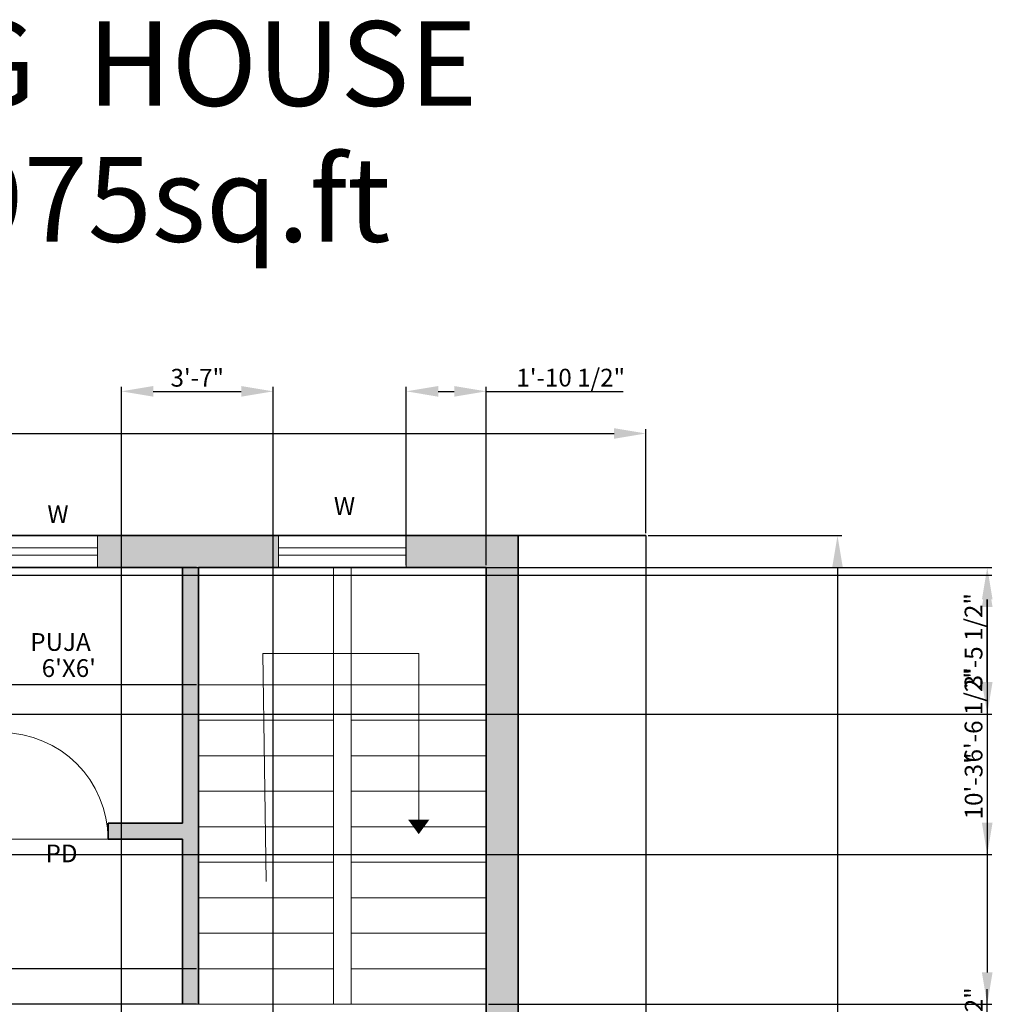
# Model space of a CAD drawing. Units: inches. Extents: x 2265 to 2807, y 1544 to 2401.
# Tile 9 of 9: x 2531 to 2807, y 2124 to 2401. Entities that reach past the tile are written whole.
import ezdxf

# ---------------------------------------------------------------- set-up
doc = ezdxf.new("R2010")
doc.units = ezdxf.units.IN
for name, color, linetype, lineweight in [('A-ANNO-DIMS', 2, 'Continuous', 18), ('A-ANNO-TEXT', 7, 'Continuous', 18), ('A-ANNO-TITL', 7, 'Continuous', 35), ('A-AREA-IDEN', 7, 'Continuous', 18), ('A-DOOR', 3, 'Continuous', 18), ('A-FLOR-STRS', 7, 'Continuous', 18), ('A-GLAZ', 4, 'Continuous', 18), ('A-WALL', 7, 'Continuous', 35), ('A-WALL-PATT', 18, 'Continuous', 13), ('C-PROP', 7, 'Continuous', 25)]:
    doc.layers.add(name, color=color, linetype=linetype, lineweight=lineweight)
doc.styles.add('ARIAL', font='times.ttf', dxfattribs={"height": 5})
doc.styles.get("Standard").update_dxf_attribs({"font": 'arial.ttf', "height": 5})
doc.dimstyles.new('ISO-25', dxfattribs={"dimtxt": 5, "dimasz": 9, "dimexe": 1.25, "dimexo": 0.625, "dimtad": 1, "dimlunit": 3, "dimtxsty": 'Standard', "dimcen": 2.5, "dimadec": 0, "dimazin": 0, "dimtfac": 1, "dimtmove": 0, "dimatfit": 3, "dimfxl": 1, "dimarcsym": 0})

# ---------------------------------------------------------------- blocks, each defined once
blk = doc.blocks.new('*D5')
at = {"layer": 'A-ANNO-DIMS', "color": 0, "lineweight": -2, "transparency": 16777216}
for p, q in [((2323.1, 2256.36), (2323.1, 2285.73)), ((2707.1, 2256.36), (2707.1, 2285.73)), ((2332.1, 2284.48), (2698.1, 2284.48))]:
    blk.add_line(p, q, dxfattribs=at)
at = {"layer": 'A-ANNO-DIMS', "color": 0, "lineweight": 100, "transparency": 16777216}
for points in [[(2332.1, 2285.98), (2332.1, 2282.98), (2323.1, 2284.48)], [(2698.1, 2285.98), (2698.1, 2282.98), (2707.1, 2284.48)]]:
    blk.add_solid(points, dxfattribs=at)
at = {"layer": 'Defpoints', "color": 0, "lineweight": 100, "transparency": 16777216}
for p in [(2707.1, 2284.48), (2323.1, 2255.73), (2707.1, 2255.73)]:
    blk.add_point(p, dxfattribs=at)
at = {"layer": 'A-ANNO-DIMS', "color": 0, "transparency": 16777216, "insert": (2515.1, 2287.66), "char_height": 5, "attachment_point": 5}
blk.add_mtext("32'", dxfattribs=at)
blk = doc.blocks.new('*D6')
at = {"layer": 'A-ANNO-DIMS', "color": 0, "lineweight": -2, "transparency": 16777216}
for p, q in [((2707.73, 2255.73), (2762.29, 2255.73)), ((2761.04, 2246.73), (2761.04, 1814.73)), ((2707.73, 1805.73), (2762.29, 1805.73))]:
    blk.add_line(p, q, dxfattribs=at)
at = {"layer": 'A-ANNO-DIMS', "color": 0, "lineweight": 100, "transparency": 16777216}
for points in [[(2759.54, 2246.73), (2762.54, 2246.73), (2761.04, 2255.73)], [(2759.54, 1814.73), (2762.54, 1814.73), (2761.04, 1805.73)]]:
    blk.add_solid(points, dxfattribs=at)
at = {"layer": 'Defpoints', "color": 0, "lineweight": 100, "transparency": 16777216}
for p in [(2707.1, 2255.73), (2707.1, 1805.73), (2761.04, 1805.73)]:
    blk.add_point(p, dxfattribs=at)
at = {"layer": 'A-ANNO-DIMS', "color": 0, "transparency": 16777216, "insert": (2757.86, 2030.73), "char_height": 5, "attachment_point": 5, "rotation": 90}
blk.add_mtext('37\'-6"', dxfattribs=at)
blk = doc.blocks.new('GLAZING-36IN')
for p, q in [((0, 36), (0, 0)), ((3.5, 36), (3.5, 0)), ((5.5, 36), (5.5, 0)), ((5.5, 36), (5.5, 0)), ((9, 0), (9, 36))]:
    blk.add_line(p, q)
blk = doc.blocks.new('GLAZING-24IN')
for p, q in [((0, 24), (0, 0)), ((3.5, 24), (3.5, 0)), ((5.5, 24), (5.5, 0)), ((5.5, 24), (5.5, 0)), ((9, 0), (9, 24))]:
    blk.add_line(p, q)
blk = doc.blocks.new('DOOR-SWING-30IN')
for p, q in [((2, 29.93), (2, 0)), ((0, 0), (30, 0))]:
    blk.add_line(p, q)
blk.add_arc((0, 0), 30, 0, 90)
blk = doc.blocks.new('*D36')
at = {"layer": 'A-ANNO-DIMS', "color": 0, "lineweight": -2, "transparency": 16777216}
for p, q in [((2662.73, 2246.73), (2804.46, 2246.73)), ((2803.21, 2237.73), (2803.21, 2132.73)), ((2662.73, 2123.73), (2804.46, 2123.73))]:
    blk.add_line(p, q, dxfattribs=at)
at = {"layer": 'A-ANNO-DIMS', "color": 0, "lineweight": 100, "transparency": 16777216}
for points in [[(2801.71, 2237.73), (2804.71, 2237.73), (2803.21, 2246.73)], [(2801.71, 2132.73), (2804.71, 2132.73), (2803.21, 2123.73)]]:
    blk.add_solid(points, dxfattribs=at)
at = {"layer": 'Defpoints', "color": 0, "lineweight": 100, "transparency": 16777216}
for p in [(2662.1, 2246.73), (2662.1, 2123.73), (2803.21, 2123.73)]:
    blk.add_point(p, dxfattribs=at)
at = {"layer": 'A-ANNO-DIMS', "color": 0, "transparency": 16777216, "insert": (2800.03, 2185.23), "char_height": 5, "attachment_point": 5, "rotation": 90}
blk.add_mtext('10\'-3"', dxfattribs=at)
blk = doc.blocks.new('*D46')
at = {"layer": 'A-ANNO-DIMS', "color": 0, "lineweight": -2, "transparency": 16777216}
for p, q in [((2803.21, 2104.95), (2803.21, 2128.02)), ((2381.23, 2095.95), (2804.46, 2095.95)), ((2803.21, 2082.06), (2803.21, 2095.95)), ((2381.23, 2082.06), (2804.46, 2082.06)), ((2803.21, 2073.06), (2803.21, 2064.06))]:
    blk.add_line(p, q, dxfattribs=at)
at = {"layer": 'A-ANNO-DIMS', "color": 0, "lineweight": 100, "transparency": 16777216}
for points in [[(2801.71, 2104.95), (2804.71, 2104.95), (2803.21, 2095.95)], [(2801.71, 2073.06), (2804.71, 2073.06), (2803.21, 2082.06)]]:
    blk.add_solid(points, dxfattribs=at)
at = {"layer": 'Defpoints', "color": 0, "lineweight": 100, "transparency": 16777216}
for p in [(2380.61, 2095.95), (2803.21, 2095.95), (2380.61, 2082.06)]:
    blk.add_point(p, dxfattribs=at)
at = {"layer": 'A-ANNO-DIMS', "color": 0, "transparency": 16777216, "insert": (2800.07, 2120.99), "char_height": 5, "attachment_point": 5, "rotation": 90}
blk.add_mtext('1\'-2"', dxfattribs=at)
blk = doc.blocks.new('*D51')
at = {"layer": 'A-ANNO-DIMS', "color": 0, "lineweight": -2, "transparency": 16777216}
for p, q in [((2470.16, 2244.62), (2804.46, 2244.62)), ((2803.21, 2235.62), (2803.21, 2174.88)), ((2466.22, 2165.88), (2804.46, 2165.88))]:
    blk.add_line(p, q, dxfattribs=at)
at = {"layer": 'A-ANNO-DIMS', "color": 0, "lineweight": 100, "transparency": 16777216}
for points in [[(2801.71, 2235.62), (2804.71, 2235.62), (2803.21, 2244.62)], [(2801.71, 2174.88), (2804.71, 2174.88), (2803.21, 2165.88)]]:
    blk.add_solid(points, dxfattribs=at)
at = {"layer": 'Defpoints', "color": 0, "lineweight": 100, "transparency": 16777216}
for p in [(2469.53, 2244.62), (2465.6, 2165.88), (2803.21, 2165.88)]:
    blk.add_point(p, dxfattribs=at)
at = {"layer": 'A-ANNO-DIMS', "color": 0, "transparency": 16777216, "insert": (2800, 2205.25), "char_height": 5, "attachment_point": 5, "rotation": 90}
blk.add_mtext('6\'-6 1/2"', dxfattribs=at)
blk = doc.blocks.new('*D52')
at = {"layer": 'A-ANNO-DIMS', "color": 0, "lineweight": -2, "transparency": 16777216}
for p, q in [((2559.35, 1939.86), (2559.35, 2297.59)), ((2568.35, 2296.34), (2593.1, 2296.34)), ((2602.1, 1939.86), (2602.1, 2297.59))]:
    blk.add_line(p, q, dxfattribs=at)
at = {"layer": 'A-ANNO-DIMS', "color": 0, "lineweight": 100, "transparency": 16777216}
for points in [[(2568.35, 2297.84), (2568.35, 2294.84), (2559.35, 2296.34)], [(2593.1, 2297.84), (2593.1, 2294.84), (2602.1, 2296.34)]]:
    blk.add_solid(points, dxfattribs=at)
at = {"layer": 'Defpoints', "color": 0, "lineweight": 100, "transparency": 16777216}
for p in [(2602.1, 2296.34), (2559.35, 1939.23), (2602.1, 1939.23)]:
    blk.add_point(p, dxfattribs=at)
at = {"layer": 'A-ANNO-DIMS', "color": 0, "transparency": 16777216, "insert": (2580.73, 2299.52), "char_height": 5, "attachment_point": 5}
blk.add_mtext('3\'-7"', dxfattribs=at)
blk = doc.blocks.new('*D56')
at = {"layer": 'A-ANNO-DIMS', "color": 0, "lineweight": -2, "transparency": 16777216}
for p, q in [((2639.6, 2247.36), (2639.6, 2297.59)), ((2648.6, 2296.34), (2653.1, 2296.34)), ((2662.1, 2247.36), (2662.1, 2297.59)), ((2662.1, 2296.34), (2700.71, 2296.34))]:
    blk.add_line(p, q, dxfattribs=at)
at = {"layer": 'A-ANNO-DIMS', "color": 0, "lineweight": 100, "transparency": 16777216}
for points in [[(2648.6, 2297.84), (2648.6, 2294.84), (2639.6, 2296.34)], [(2653.1, 2297.84), (2653.1, 2294.84), (2662.1, 2296.34)]]:
    blk.add_solid(points, dxfattribs=at)
at = {"layer": 'Defpoints', "color": 0, "lineweight": 100, "transparency": 16777216}
for p in [(2662.1, 2296.34), (2639.6, 2246.73), (2662.1, 2246.73)]:
    blk.add_point(p, dxfattribs=at)
at = {"layer": 'A-ANNO-DIMS', "color": 0, "transparency": 16777216, "insert": (2685.9, 2299.55), "char_height": 5, "attachment_point": 5}
blk.add_mtext('1\'-10 1/2"', dxfattribs=at)
blk = doc.blocks.new('*D57')
at = {"layer": 'A-ANNO-DIMS', "color": 0, "lineweight": -2, "transparency": 16777216}
for p, q in [((2368.73, 2246.73), (2804.46, 2246.73)), ((2803.21, 2214.48), (2803.21, 2237.73)), ((2368.73, 2205.48), (2804.46, 2205.48))]:
    blk.add_line(p, q, dxfattribs=at)
at = {"layer": 'A-ANNO-DIMS', "color": 0, "lineweight": 100, "transparency": 16777216}
for points in [[(2801.71, 2237.73), (2804.71, 2237.73), (2803.21, 2246.73)], [(2801.71, 2214.48), (2804.71, 2214.48), (2803.21, 2205.48)]]:
    blk.add_solid(points, dxfattribs=at)
at = {"layer": 'Defpoints', "color": 0, "lineweight": 100, "transparency": 16777216}
for p in [(2368.1, 2246.73), (2803.21, 2246.73), (2368.1, 2205.48)]:
    blk.add_point(p, dxfattribs=at)
at = {"layer": 'A-ANNO-DIMS', "color": 0, "transparency": 16777216, "insert": (2800, 2226.11), "char_height": 5, "attachment_point": 5, "rotation": 90}
blk.add_mtext('3\'-5 1/2"', dxfattribs=at)
blk = doc.blocks.new('*D59')
at = {"layer": 'A-ANNO-DIMS', "color": 0, "lineweight": -2, "transparency": 16777216}
for p, q in [((2580.48, 2246.73), (2274.04, 2246.73)), ((2275.29, 2237.73), (2275.29, 2222.73)), ((2580.48, 2213.73), (2274.04, 2213.73))]:
    blk.add_line(p, q, dxfattribs=at)
at = {"layer": 'A-ANNO-DIMS', "color": 0, "lineweight": 100, "transparency": 16777216}
for points in [[(2273.79, 2237.73), (2276.79, 2237.73), (2275.29, 2246.73)], [(2273.79, 2222.73), (2276.79, 2222.73), (2275.29, 2213.73)]]:
    blk.add_solid(points, dxfattribs=at)
at = {"layer": 'Defpoints', "color": 0, "lineweight": 100, "transparency": 16777216}
for p in [(2581.1, 2246.73), (2275.29, 2213.73), (2581.1, 2213.73)]:
    blk.add_point(p, dxfattribs=at)
at = {"layer": 'A-ANNO-DIMS', "color": 0, "transparency": 16777216, "insert": (2272.11, 2230.23), "char_height": 5, "attachment_point": 5, "rotation": 90}
blk.add_mtext('2\'-9"', dxfattribs=at)
blk = doc.blocks.new('*D60')
at = {"layer": 'A-ANNO-DIMS', "color": 0, "lineweight": -2, "transparency": 16777216}
for p, q in [((2275.29, 2142.73), (2275.29, 2151.73)), ((2580.48, 2133.73), (2274.04, 2133.73)), ((2275.29, 2133.73), (2275.29, 2123.73)), ((2580.48, 2123.73), (2274.04, 2123.73)), ((2275.29, 2114.73), (2275.29, 2087.31))]:
    blk.add_line(p, q, dxfattribs=at)
at = {"layer": 'A-ANNO-DIMS', "color": 0, "lineweight": 100, "transparency": 16777216}
for points in [[(2273.79, 2142.73), (2276.79, 2142.73), (2275.29, 2133.73)], [(2273.79, 2114.73), (2276.79, 2114.73), (2275.29, 2123.73)]]:
    blk.add_solid(points, dxfattribs=at)
at = {"layer": 'Defpoints', "color": 0, "lineweight": 100, "transparency": 16777216}
for p in [(2581.1, 2133.73), (2275.29, 2123.73), (2581.1, 2123.73)]:
    blk.add_point(p, dxfattribs=at)
at = {"layer": 'A-ANNO-DIMS', "color": 0, "transparency": 16777216, "insert": (2272.11, 2096.52), "char_height": 5, "attachment_point": 5, "rotation": 90}
blk.add_mtext('0\'-10"', dxfattribs=at)

msp = doc.modelspace()

# ---------------------------------------------------------------- hatches: boundary and pattern name
at = {"layer": 'A-WALL-PATT'}
h = msp.add_hatch(color=256, dxfattribs=at)
h.dxf.hatch_style = 1
h.paths.add_polyline_path([(2416.101, 2255.733), (2359.101, 2255.733), (2359.101, 2205.483), (2368.101, 2205.483), (2368.101, 2246.733), (2416.101, 2246.733)])
h.paths.add_polyline_path([(2528.601, 2255.733), (2452.101, 2255.733), (2452.101, 2246.733), (2487.251, 2246.733), (2500.101, 2246.733), (2500.101, 2168.733), (2504.601, 2168.733), (2504.601, 2170.233), (2525.601, 2170.233), (2525.601, 2174.733), (2504.601, 2174.733), (2504.601, 2246.733), (2528.601, 2246.733)])
h.paths.add_polyline_path([(2603.601, 2255.733), (2552.601, 2255.733), (2552.601, 2246.733), (2576.601, 2246.733), (2576.601, 2174.733), (2555.601, 2174.733), (2555.601, 2170.233), (2576.601, 2170.233), (2576.601, 2123.733), (2581.101, 2123.733), (2581.101, 2246.733), (2603.601, 2246.733)])
h.paths.add_polyline_path([(2671.101, 2255.733), (2639.601, 2255.733), (2639.601, 2246.733), (2662.101, 2246.733), (2662.101, 2083.435), (2671.101, 2083.435)])
h.paths.add_polyline_path([(2671.101, 2035.435), (2662.101, 2035.435), (2662.101, 1939.233), (2644.101, 1939.233), (2644.101, 1930.233), (2662.101, 1930.233), (2662.101, 1814.733), (2644.101, 1814.733), (2644.101, 1805.733), (2671.101, 1805.733)])
h.paths.add_polyline_path([(2368.101, 1930.233), (2511.351, 1930.233), (2511.351, 1939.233), (2468.601, 1939.233), (2468.601, 2032.233), (2464.101, 2032.233), (2464.101, 1939.233), (2368.101, 1939.233), (2368.101, 1995.884), (2359.101, 1995.884), (2359.101, 1805.733), (2602.101, 1805.733), (2602.101, 1814.733), (2368.101, 1814.733)])
h.paths.add_polyline_path([(2368.101, 2071.233), (2464.101, 2071.233), (2464.101, 2062.233), (2468.601, 2062.233), (2468.601, 2123.733), (2504.601, 2123.733), (2504.601, 2132.733), (2500.101, 2132.733), (2500.101, 2128.233), (2455.101, 2128.233), (2455.101, 2123.733), (2464.101, 2123.733), (2464.101, 2075.733), (2368.101, 2075.733), (2368.101, 2087.733), (2359.101, 2087.733), (2359.101, 2031.884), (2368.101, 2031.884)])
h.paths.add_polyline_path([(2368.101, 2169.483), (2359.101, 2169.483), (2359.101, 2111.733), (2368.101, 2111.733), (2368.101, 2123.733), (2425.101, 2123.733), (2425.101, 2128.233), (2368.101, 2128.233)])

# ---------------------------------------------------------------- linework, layer by layer
at = {"layer": 'A-FLOR-STRS'}
for p, q in [((2619.101, 2123.733), (2619.101, 2246.733)), ((2624.101, 2246.733), (2624.101, 2123.733)), ((2624.101, 2246.733), (2624.101, 2123.733)), ((2600.101, 2158.354), (2599.232, 2222.551)), ((2599.232, 2222.551), (2643.101, 2222.551)), ((2643.101, 2222.551), (2643.101, 2175.737)), ((2662.101, 2213.733), (2581.101, 2213.733)), ((2619.101, 2203.733), (2581.101, 2203.733)), ((2662.101, 2203.733), (2624.101, 2203.733)), ((2619.101, 2193.733), (2581.101, 2193.733)), ((2662.101, 2193.733), (2624.101, 2193.733)), ((2619.101, 2183.733), (2581.101, 2183.733)), ((2662.101, 2183.733), (2624.101, 2183.733)), ((2619.101, 2173.733), (2581.101, 2173.733)), ((2662.101, 2173.733), (2624.101, 2173.733)), ((2619.101, 2163.733), (2581.101, 2163.733)), ((2662.101, 2163.733), (2624.101, 2163.733)), ((2619.101, 2153.733), (2581.101, 2153.733)), ((2662.101, 2153.733), (2624.101, 2153.733)), ((2619.101, 2143.733), (2581.101, 2143.733)), ((2662.101, 2143.733), (2624.101, 2143.733)), ((2619.101, 2133.733), (2581.101, 2133.733)), ((2662.101, 2133.733), (2624.101, 2133.733)), ((2662.101, 2123.733), (2576.601, 2123.733))]:
    msp.add_line(p, q, dxfattribs=at)
msp.add_lwpolyline([(2643.101, 2175.737, 6, 0, 0), (2643.101, 2171.639, 0, 0, 0)], format="xyseb", dxfattribs=at)
at = {"layer": 'A-GLAZ'}
for p, q in [((2552.601, 2246.733), (2552.601, 2255.733)), ((2603.601, 2255.733), (2603.601, 2246.733)), ((2639.601, 2246.733), (2639.601, 2255.733))]:
    msp.add_line(p, q, dxfattribs=at)
at = {"layer": 'A-WALL'}
for p, q in [((2323.101, 2255.733), (2707.101, 2255.733)), ((2671.101, 2255.733), (2671.101, 1805.733)), ((2504.601, 2246.733), (2576.601, 2246.733)), ((2576.601, 2174.733), (2576.601, 2246.733)), ((2581.101, 2123.733), (2581.101, 2246.733)), ((2581.101, 2246.733), (2662.101, 2246.733)), ((2662.101, 2246.733), (2662.101, 1939.233)), ((2555.601, 2174.733), (2555.601, 2170.233)), ((2555.601, 2174.733), (2576.601, 2174.733)), ((2555.601, 2170.233), (2576.601, 2170.233)), ((2576.601, 2123.733), (2576.601, 2170.233))]:
    msp.add_line(p, q, dxfattribs=at)
at = {"layer": 'C-PROP'}
msp.add_line((2707.101, 2255.733), (2707.101, 1805.733), dxfattribs=at)

# ---------------------------------------------------------------- block references
at = {"layer": 'A-DOOR'}
msp.add_blockref('DOOR-SWING-30IN', (2525.601, 2170.233), dxfattribs=at)
at = {"layer": 'A-GLAZ'}
for name, p, rotation in [('GLAZING-24IN', (2552.601, 2246.733), 89.9999999999955), ('GLAZING-36IN', (2639.601, 2246.733), 89.99999999999694)]:
    msp.add_blockref(name, p, dxfattribs=dict(at, rotation=rotation))

# ---------------------------------------------------------------- texts
at = {"layer": 'A-ANNO-TEXT', "style": 'ARIAL'}
for s, p in [('W', (2619.203, 2261.556)), ('W', (2538.51, 2259.272)), ('PD', (2538.001, 2163.723))]:
    msp.add_text(s, height=5, dxfattribs=at).set_placement(p)
at = {"layer": 'A-ANNO-TITL'}
for s, p in [('EAST FACING  HOUSE', (2336.336, 2376.748)), ('           AREA=975sq.ft', (2336.336, 2338.469))]:
    msp.add_text(s, height=23.82874, dxfattribs=at).set_placement(p)
at = {"layer": 'A-AREA-IDEN', "style": 'ARIAL'}
for s, p in [('PUJA', (2533.702, 2223.26)), ("6'X6'", (2536.919, 2215.911))]:
    msp.add_text(s, height=5, dxfattribs=at).set_placement(p)

# ---------------------------------------------------------------- dimensions: what is measured, and where the dimension line sits
at = {"layer": 'A-ANNO-DIMS'}
for base, p1, p2, override, picture, middle in [((2662.101, 2296.343), (2639.601, 2246.733), (2662.101, 2246.733), {"dimdec": 1, "dimlfac": 1, "dimrnd": 0, "dimzin": 1, "dimdsep": 46, "dimlunit": 4, "dimfrac": 2}, '*D56', (2685.904, 2299.554)), ((2602.101182, 2296.343269), (2559.351182, 1939.233269), (2602.101182, 1939.233269), {"dimdec": 1, "dimlfac": 1, "dimrnd": 0, "dimzin": 1, "dimdsep": 46, "dimlunit": 4, "dimfrac": 2}, '*D52', (2580.726182, 2299.522839259)), ((2707.101, 2284.48), (2323.101, 2255.733), (2707.101, 2255.733), {"dimclrd": 0, "dimclre": 0, "dimclrt": 0}, '*D5', (2515.101, 2287.659))]:
    dim = msp.add_linear_dim(base=base, p1=p1, p2=p2, dimstyle='ISO-25', override=override, dxfattribs=at)
    dim.commit()
    dim.dimension.update_dxf_attribs({"geometry": picture, "text_midpoint": middle})
for base, p1, p2, override, picture, middle in [((2761.041, 1805.733), (2707.101, 2255.733), (2707.101, 1805.733), {"dimclrd": 0, "dimclre": 0, "dimclrt": 0}, '*D6', (2757.861, 2030.733)), ((2275.289, 2213.733), (2581.101, 2246.733), (2581.101, 2213.733), {"dimdec": 1, "dimlfac": 1, "dimrnd": 0, "dimzin": 1, "dimdsep": 46, "dimlunit": 4, "dimfrac": 2}, '*D59', (2272.111, 2230.233)), ((2803.210028, 2246.733269), (2368.101182, 2205.483269), (2368.101182, 2246.733269), {"dimdec": 1, "dimlfac": 1, "dimrnd": 0, "dimzin": 1, "dimdsep": 46, "dimlunit": 4, "dimfrac": 2}, '*D57', (2799.998056649, 2226.108269)), ((2803.21, 2123.733), (2662.101, 2246.733), (2662.101, 2123.733), {"dimdec": 1, "dimlfac": 1, "dimrnd": 0, "dimzin": 1, "dimdsep": 46, "dimlunit": 4, "dimfrac": 2}, '*D36', (2800.03, 2185.233)), ((2803.21, 2165.875), (2469.534, 2244.615), (2465.597, 2165.875), {"dimdec": 1, "dimlfac": 1, "dimrnd": 0, "dimzin": 1, "dimdsep": 46, "dimlunit": 4, "dimfrac": 2}, '*D51', (2800, 2205.245)), ((2275.289, 2123.733), (2581.101, 2133.733), (2581.101, 2123.733), {"dimdec": 1, "dimlfac": 1, "dimrnd": 0, "dimzin": 1, "dimdsep": 46, "dimlunit": 4, "dimfrac": 2}, '*D60', (2272.111, 2096.52)), ((2803.21, 2095.951), (2380.607, 2082.055), (2380.607, 2095.951), {"dimdec": 1, "dimlfac": 1, "dimrnd": 0, "dimzin": 1, "dimdsep": 46, "dimlunit": 4, "dimfrac": 2}, '*D46', (2800.075, 2120.986))]:
    dim = msp.add_linear_dim(base=base, p1=p1, p2=p2, angle=90, dimstyle='ISO-25', override=override, dxfattribs=at)
    dim.commit()
    dim.dimension.update_dxf_attribs({"geometry": picture, "text_midpoint": middle})

doc.saveas('drawing.dxf')
